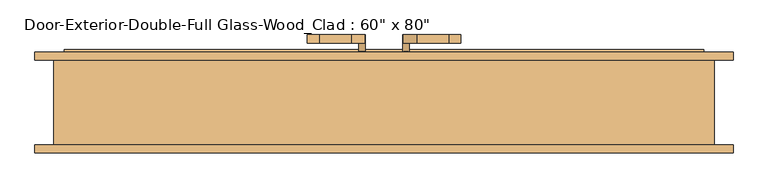
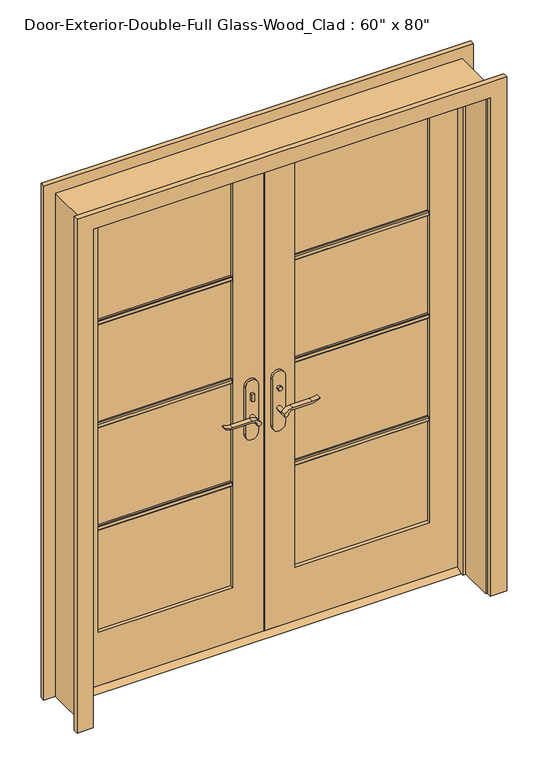
"""IFC4 building model written with IfcOpenShell, lengths in millimetres: door geometry."""

from ifc_helpers import new_model, si_unit, point, frame, frame_2d, origin, place, context, project, spatial, polyline, circle_curve, trimmed, segment, composite_curve, outline, extrude, faceted_brep, source, transform, mapped, element, save


def door_b03bd389(model_context):
    return source(origin(), model_context, "Body", "SolidModel", [
        extrude(outline(polyline([(63.5, 12.7), (98.425, 12.7), (123.825, 0.0), (38.1, 0.0), (63.5, 12.7)])), frame((-762.0, 0.0, 0.0), z_axis=(1.0, 0.0, 0.0), x_axis=(0.0, 1.0, 0.0)), (0.0, 0.0, 1.0), 1524.0),
        extrude(outline(polyline([(-47.4019111, 43.5), (-57.4019111, 43.5), (-57.4019111, 53.5), (-47.4019111, 53.5), (-47.4019111, 43.5)])), frame((0.0, 0.0, 981.9), z_axis=(0.0, 0.0, 1.0), x_axis=(1.0, 0.0, 0.0)), (0.0, 0.0, 1.0), 30.0),
        extrude(outline(composite_curve([segment(trimmed(circle_curve(frame_2d((996.9, -52.4019111)), 8.0), [point((996.9, -60.4019111))], [point((996.9, -44.4019111))], False, "CARTESIAN"), True, "CONTINUOUS"), segment(trimmed(circle_curve(frame_2d((996.9, -52.4019111)), 8.0), [point((996.9, -44.4019111))], [point((996.9, -60.4019111))], False, "CARTESIAN"), True, "CONTINUOUS")], self_intersect=False)), frame((0.0, 108.425, 0.0), z_axis=(0.0, 1.0, 0.0), x_axis=(0.0, 0.0, 1.0)), (0.0, 0.0, 1.0), 10.0),
        extrude(outline(composite_curve([segment(trimmed(circle_curve(frame_2d((897.1555521, -76.0694241)), 37.2832219), [point((919.0523287, -45.8937749))], [point((934.4, -77.7693445))], False, "CARTESIAN"), True, "CONTINUOUS"), segment(polyline([(934.4, -77.7693445), (934.4, -154.045502)]), True, "CONTINUOUS"), segment(trimmed(circle_curve(frame_2d((1017.6850638, -153.9791202)), 83.2850902), [point((934.4, -154.045502))], [point((939.4, -182.4019111))], True, "CARTESIAN"), True, "CONTINUOUS"), segment(polyline([(939.4, -182.4019111), (936.6135558, -182.4019111)]), True, "CONTINUOUS"), segment(trimmed(circle_curve(frame_2d((986.6709207, -150.4622499)), 59.3791355), [point((936.6135558, -182.4019111))], [point((927.4, -154.045502))], False, "CARTESIAN"), True, "CONTINUOUS"), segment(polyline([(927.4, -154.045502), (927.4, -77.7881013)]), True, "CONTINUOUS"), segment(trimmed(circle_curve(frame_2d((909.2738613, -77.7881013)), 18.1261387), [point((927.4, -77.7881013))], [point((914.4, -60.4019111))], True, "CARTESIAN"), True, "CONTINUOUS"), segment(trimmed(circle_curve(frame_2d((914.4, -52.4019111)), 8.0), [point((914.4, -60.4019111))], [point((919.0523287, -45.8937749))], False, "CARTESIAN"), True, "CONTINUOUS")], self_intersect=False)), frame((0.0, 3.5, 0.0), z_axis=(0.0, 1.0, 0.0), x_axis=(0.0, 0.0, 1.0)), (0.0, 0.0, 1.0), 20.0),
        extrude(outline(composite_curve([segment(trimmed(circle_curve(frame_2d((914.4, -52.4019111)), 8.0), [point((914.3999903, -60.4019111))], [point((919.0523287, -45.8937749))], False, "CARTESIAN"), True, "CONTINUOUS"), segment(trimmed(circle_curve(frame_2d((897.1555521, -76.0694241)), 37.2832219), [point((919.0523287, -45.8937749))], [point((934.4, -77.7693445))], False, "CARTESIAN"), True, "CONTINUOUS"), segment(polyline([(934.4, -77.7693445), (934.4, -154.045502)]), True, "CONTINUOUS"), segment(trimmed(circle_curve(frame_2d((1017.6850638, -153.9791202)), 83.2850902), [point((934.4, -154.045502))], [point((939.4, -182.4019111))], True, "CARTESIAN"), True, "CONTINUOUS"), segment(polyline([(939.4, -182.4019111), (936.6135558, -182.4019111)]), True, "CONTINUOUS"), segment(trimmed(circle_curve(frame_2d((986.6709207, -150.4622499)), 59.3791355), [point((936.6135558, -182.4019111))], [point((927.4, -154.045502))], False, "CARTESIAN"), True, "CONTINUOUS"), segment(polyline([(927.4, -154.045502), (927.4, -77.788099)]), True, "CONTINUOUS"), segment(trimmed(circle_curve(frame_2d((909.2738682, -77.788099)), 18.1261318), [point((927.4, -77.788099))], [point((914.3999903, -60.4019111))], True, "CARTESIAN"), True, "CONTINUOUS")], self_intersect=False)), frame((0.0, 138.425, 0.0), z_axis=(0.0, 1.0, 0.0), x_axis=(0.0, 0.0, 1.0)), (0.0, 0.0, 1.0), 20.0),
        extrude(outline(composite_curve([segment(trimmed(circle_curve(frame_2d((914.4, -52.4019111)), 8.0), [point((914.4, -60.4019111))], [point((914.4, -44.4019111))], False, "CARTESIAN"), True, "CONTINUOUS"), segment(trimmed(circle_curve(frame_2d((914.4, -52.4019111)), 8.0), [point((914.4, -44.4019111))], [point((914.4, -60.4019111))], False, "CARTESIAN"), True, "CONTINUOUS")], self_intersect=False)), frame((0.0, 23.5, 0.0), z_axis=(0.0, 1.0, 0.0), x_axis=(0.0, 0.0, 1.0)), (0.0, 0.0, 1.0), 30.0),
        extrude(outline(composite_curve([segment(trimmed(circle_curve(frame_2d((914.4, -52.4019111)), 8.0), [point((914.4, -60.4019111))], [point((914.4, -44.4019111))], False, "CARTESIAN"), True, "CONTINUOUS"), segment(trimmed(circle_curve(frame_2d((914.4, -52.4019111)), 8.0), [point((914.4, -44.4019111))], [point((914.4, -60.4019111))], False, "CARTESIAN"), True, "CONTINUOUS")], self_intersect=False)), frame((0.0, 108.425, 0.0), z_axis=(0.0, 1.0, 0.0), x_axis=(0.0, 0.0, 1.0)), (0.0, 0.0, 1.0), 30.0),
        extrude(outline(composite_curve([segment(polyline([(844.4, -27.4019111), (1039.4, -27.4019111)]), True, "CONTINUOUS"), segment(trimmed(circle_curve(frame_2d((1039.4, -52.4019111)), 25.0), [point((1039.4, -27.4019111))], [point((1039.4, -77.4019111))], False, "CARTESIAN"), True, "CONTINUOUS"), segment(polyline([(1039.4, -77.4019111), (844.4, -77.4019111)]), True, "CONTINUOUS"), segment(trimmed(circle_curve(frame_2d((844.4, -52.4019111)), 25.0), [point((844.4, -77.4019111))], [point((844.4, -27.4019111))], False, "CARTESIAN"), True, "CONTINUOUS")], self_intersect=False)), frame((0.0, 53.5, 0.0), z_axis=(0.0, 1.0, 0.0), x_axis=(0.0, 0.0, 1.0)), (0.0, 0.0, 1.0), 10.0),
        extrude(outline(composite_curve([segment(polyline([(844.4, -27.4019111), (1039.4, -27.4019111)]), True, "CONTINUOUS"), segment(trimmed(circle_curve(frame_2d((1039.4, -52.4019111)), 25.0), [point((1039.4, -27.4019111))], [point((1039.4, -77.4019111))], False, "CARTESIAN"), True, "CONTINUOUS"), segment(polyline([(1039.4, -77.4019111), (844.4, -77.4019111)]), True, "CONTINUOUS"), segment(trimmed(circle_curve(frame_2d((844.4, -52.4019111)), 25.0), [point((844.4, -77.4019111))], [point((844.4, -27.4019111))], False, "CARTESIAN"), True, "CONTINUOUS")], self_intersect=False)), frame((0.0, 98.425, 0.0), z_axis=(0.0, 1.0, 0.0), x_axis=(0.0, 0.0, 1.0)), (0.0, 0.0, 1.0), 10.0),
        extrude(outline(polyline([(47.3875, 118.425), (57.3875, 118.425), (57.3875, 108.425), (47.3875, 108.425), (47.3875, 118.425)])), frame((0.0, 0.0, 981.9), z_axis=(0.0, 0.0, 1.0), x_axis=(1.0, 0.0, 0.0)), (0.0, 0.0, 1.0), 30.0),
        extrude(outline(composite_curve([segment(trimmed(circle_curve(frame_2d((996.9, 52.3875)), 8.0), [point((996.9, 60.3875))], [point((996.9, 44.3875))], False, "CARTESIAN"), True, "CONTINUOUS"), segment(trimmed(circle_curve(frame_2d((996.9, 52.3875)), 8.0), [point((996.9, 44.3875))], [point((996.9, 60.3875))], False, "CARTESIAN"), True, "CONTINUOUS")], self_intersect=False)), frame((0.0, 43.5, 0.0), z_axis=(0.0, 1.0, 0.0), x_axis=(0.0, 0.0, 1.0)), (0.0, 0.0, 1.0), 10.0),
        extrude(outline(composite_curve([segment(trimmed(circle_curve(frame_2d((914.4, 52.3875)), 8.0), [point((919.0523287, 45.8793637))], [point((914.4, 60.3875))], False, "CARTESIAN"), True, "CONTINUOUS"), segment(trimmed(circle_curve(frame_2d((909.2738613, 77.7736901)), 18.1261387), [point((914.4, 60.3875))], [point((927.4, 77.7736901))], True, "CARTESIAN"), True, "CONTINUOUS"), segment(polyline([(927.4, 77.7736901), (927.4, 154.0310909)]), True, "CONTINUOUS"), segment(trimmed(circle_curve(frame_2d((986.6709207, 150.4478388)), 59.3791355), [point((927.4, 154.0310909))], [point((936.6135558, 182.3875))], False, "CARTESIAN"), True, "CONTINUOUS"), segment(polyline([(936.6135558, 182.3875), (939.4, 182.3875)]), True, "CONTINUOUS"), segment(trimmed(circle_curve(frame_2d((1017.6850638, 153.9647091)), 83.2850902), [point((939.4, 182.3875))], [point((934.4, 154.0310909))], True, "CARTESIAN"), True, "CONTINUOUS"), segment(polyline([(934.4, 154.0310909), (934.4, 77.7549333)]), True, "CONTINUOUS"), segment(trimmed(circle_curve(frame_2d((897.1555521, 76.0550129)), 37.2832219), [point((934.4, 77.7549333))], [point((919.0523287, 45.8793637))], False, "CARTESIAN"), True, "CONTINUOUS")], self_intersect=False)), frame((0.0, 138.425, 0.0), z_axis=(0.0, 1.0, 0.0), x_axis=(0.0, 0.0, 1.0)), (0.0, 0.0, 1.0), 20.0),
        extrude(outline(composite_curve([segment(trimmed(circle_curve(frame_2d((909.2738682, 77.7736878)), 18.1261318), [point((914.3999903, 60.3875))], [point((927.4, 77.7736878))], True, "CARTESIAN"), True, "CONTINUOUS"), segment(polyline([(927.4, 77.7736878), (927.4, 154.0310909)]), True, "CONTINUOUS"), segment(trimmed(circle_curve(frame_2d((986.6709207, 150.4478388)), 59.3791355), [point((927.4, 154.0310909))], [point((936.6135558, 182.3875))], False, "CARTESIAN"), True, "CONTINUOUS"), segment(polyline([(936.6135558, 182.3875), (939.4, 182.3875)]), True, "CONTINUOUS"), segment(trimmed(circle_curve(frame_2d((1017.6850638, 153.9647091)), 83.2850902), [point((939.4, 182.3875))], [point((934.4, 154.0310909))], True, "CARTESIAN"), True, "CONTINUOUS"), segment(polyline([(934.4, 154.0310909), (934.4, 77.7549333)]), True, "CONTINUOUS"), segment(trimmed(circle_curve(frame_2d((897.1555521, 76.0550129)), 37.2832219), [point((934.4, 77.7549333))], [point((919.0523287, 45.8793637))], False, "CARTESIAN"), True, "CONTINUOUS"), segment(trimmed(circle_curve(frame_2d((914.4, 52.3875)), 8.0), [point((919.0523287, 45.8793637))], [point((914.3999903, 60.3875))], False, "CARTESIAN"), True, "CONTINUOUS")], self_intersect=False)), frame((0.0, 3.5, 0.0), z_axis=(0.0, 1.0, 0.0), x_axis=(0.0, 0.0, 1.0)), (0.0, 0.0, 1.0), 20.0),
        extrude(outline(composite_curve([segment(trimmed(circle_curve(frame_2d((914.4, 52.3875)), 8.0), [point((914.4, 60.3875))], [point((914.4, 44.3875))], False, "CARTESIAN"), True, "CONTINUOUS"), segment(trimmed(circle_curve(frame_2d((914.4, 52.3875)), 8.0), [point((914.4, 44.3875))], [point((914.4, 60.3875))], False, "CARTESIAN"), True, "CONTINUOUS")], self_intersect=False)), frame((0.0, 108.425, 0.0), z_axis=(0.0, 1.0, 0.0), x_axis=(0.0, 0.0, 1.0)), (0.0, 0.0, 1.0), 30.0),
        extrude(outline(composite_curve([segment(trimmed(circle_curve(frame_2d((914.4, 52.3875)), 8.0), [point((914.4, 60.3875))], [point((914.4, 44.3875))], False, "CARTESIAN"), True, "CONTINUOUS"), segment(trimmed(circle_curve(frame_2d((914.4, 52.3875)), 8.0), [point((914.4, 44.3875))], [point((914.4, 60.3875))], False, "CARTESIAN"), True, "CONTINUOUS")], self_intersect=False)), frame((0.0, 23.5, 0.0), z_axis=(0.0, 1.0, 0.0), x_axis=(0.0, 0.0, 1.0)), (0.0, 0.0, 1.0), 30.0),
        extrude(outline(composite_curve([segment(trimmed(circle_curve(frame_2d((844.4, 52.3875)), 25.0), [point((844.4, 27.3875))], [point((844.4, 77.3875))], False, "CARTESIAN"), True, "CONTINUOUS"), segment(polyline([(844.4, 77.3875), (1039.4, 77.3875)]), True, "CONTINUOUS"), segment(trimmed(circle_curve(frame_2d((1039.4, 52.3875)), 25.0), [point((1039.4, 77.3875))], [point((1039.4, 27.3875))], False, "CARTESIAN"), True, "CONTINUOUS"), segment(polyline([(1039.4, 27.3875), (844.4, 27.3875)]), True, "CONTINUOUS")], self_intersect=False)), frame((0.0, 98.425, 0.0), z_axis=(0.0, 1.0, 0.0), x_axis=(0.0, 0.0, 1.0)), (0.0, 0.0, 1.0), 10.0),
        extrude(outline(composite_curve([segment(trimmed(circle_curve(frame_2d((844.4, 52.3875)), 25.0), [point((844.4, 27.3875))], [point((844.4, 77.3875))], False, "CARTESIAN"), True, "CONTINUOUS"), segment(polyline([(844.4, 77.3875), (1039.4, 77.3875)]), True, "CONTINUOUS"), segment(trimmed(circle_curve(frame_2d((1039.4, 52.3875)), 25.0), [point((1039.4, 77.3875))], [point((1039.4, 27.3875))], False, "CARTESIAN"), True, "CONTINUOUS"), segment(polyline([(1039.4, 27.3875), (844.4, 27.3875)]), True, "CONTINUOUS")], self_intersect=False)), frame((0.0, 53.5, 0.0), z_axis=(0.0, 1.0, 0.0), x_axis=(0.0, 0.0, 1.0)), (0.0, 0.0, 1.0), 10.0),
        extrude(outline(polyline([(77.47, 1502.171875), (77.47, 1483.121875), (71.12, 1483.121875), (67.945, 1486.296875), (67.945, 1498.996875), (71.12, 1502.171875), (77.47, 1502.171875)])), frame((120.65, 0.0, 0.0), z_axis=(1.0, 0.0, 0.0), x_axis=(0.0, 1.0, 0.0)), (0.0, 0.0, 1.0), 520.7),
        extrude(outline(polyline([(77.47, 1081.88125), (77.47, 1062.83125), (71.12, 1062.83125), (67.945, 1066.00625), (67.945, 1078.70625), (71.12, 1081.88125), (77.47, 1081.88125)])), frame((120.65, 0.0, 0.0), z_axis=(1.0, 0.0, 0.0), x_axis=(0.0, 1.0, 0.0)), (0.0, 0.0, 1.0), 520.7),
        extrude(outline(polyline([(77.47, 661.590625), (77.47, 642.540625), (71.12, 642.540625), (67.945, 645.715625), (67.945, 658.415625), (71.12, 661.590625), (77.47, 661.590625)])), frame((120.65, 0.0, 0.0), z_axis=(1.0, 0.0, 0.0), x_axis=(0.0, 1.0, 0.0)), (0.0, 0.0, 1.0), 520.7),
        extrude(outline(polyline([(84.455, 1502.171875), (90.805, 1502.171875), (93.98, 1498.996875), (93.98, 1486.296875), (90.805, 1483.121875), (84.455, 1483.121875), (84.455, 1502.171875)])), frame((-641.35, 0.0, 0.0), z_axis=(1.0, 0.0, 0.0), x_axis=(0.0, 1.0, 0.0)), (0.0, 0.0, 1.0), 520.7),
        extrude(outline(polyline([(84.455, 1081.88125), (90.805, 1081.88125), (93.98, 1078.70625), (93.98, 1066.00625), (90.805, 1062.83125), (84.455, 1062.83125), (84.455, 1081.88125)])), frame((-641.35, 0.0, 0.0), z_axis=(1.0, 0.0, 0.0), x_axis=(0.0, 1.0, 0.0)), (0.0, 0.0, 1.0), 520.7),
        extrude(outline(polyline([(84.455, 661.590625), (90.805, 661.590625), (93.98, 658.415625), (93.98, 645.715625), (90.805, 642.540625), (84.455, 642.540625), (84.455, 661.590625)])), frame((-641.35, 0.0, 0.0), z_axis=(1.0, 0.0, 0.0), x_axis=(0.0, 1.0, 0.0)), (0.0, 0.0, 1.0), 520.7),
        extrude(outline(polyline([(84.455, 1502.171875), (90.805, 1502.171875), (93.98, 1498.996875), (93.98, 1486.296875), (90.805, 1483.121875), (84.455, 1483.121875), (84.455, 1502.171875)])), frame((120.65, 0.0, 0.0), z_axis=(1.0, 0.0, 0.0), x_axis=(0.0, 1.0, 0.0)), (0.0, 0.0, 1.0), 520.7),
        extrude(outline(polyline([(84.455, 1081.88125), (90.805, 1081.88125), (93.98, 1078.70625), (93.98, 1066.00625), (90.805, 1062.83125), (84.455, 1062.83125), (84.455, 1081.88125)])), frame((120.65, 0.0, 0.0), z_axis=(1.0, 0.0, 0.0), x_axis=(0.0, 1.0, 0.0)), (0.0, 0.0, 1.0), 520.7),
        extrude(outline(polyline([(84.455, 661.590625), (90.805, 661.590625), (93.98, 658.415625), (93.98, 645.715625), (90.805, 642.540625), (84.455, 642.540625), (84.455, 661.590625)])), frame((120.65, 0.0, 0.0), z_axis=(1.0, 0.0, 0.0), x_axis=(0.0, 1.0, 0.0)), (0.0, 0.0, 1.0), 520.7),
        extrude(outline(polyline([(77.47, 1502.171875), (77.47, 1483.121875), (71.12, 1483.121875), (67.945, 1486.296875), (67.945, 1498.996875), (71.12, 1502.171875), (77.47, 1502.171875)])), frame((-641.35, 0.0, 0.0), z_axis=(1.0, 0.0, 0.0), x_axis=(0.0, 1.0, 0.0)), (0.0, 0.0, 1.0), 520.7),
        extrude(outline(polyline([(77.47, 1081.88125), (77.47, 1062.83125), (71.12, 1062.83125), (67.945, 1066.00625), (67.945, 1078.70625), (71.12, 1081.88125), (77.47, 1081.88125)])), frame((-641.35, 0.0, 0.0), z_axis=(1.0, 0.0, 0.0), x_axis=(0.0, 1.0, 0.0)), (0.0, 0.0, 1.0), 520.7),
        extrude(outline(polyline([(77.47, 661.590625), (77.47, 642.540625), (71.12, 642.540625), (67.945, 645.715625), (67.945, 658.415625), (71.12, 661.590625), (77.47, 661.590625)])), frame((-641.35, 0.0, 0.0), z_axis=(1.0, 0.0, 0.0), x_axis=(0.0, 1.0, 0.0)), (0.0, 0.0, 1.0), 520.7),
        extrude(outline(polyline([(0.0, 768.35), (0.0, 831.85), (2101.85, 831.85), (2101.85, -831.85), (0.0, -831.85), (0.0, -768.35), (2038.35, -768.35), (2038.35, 768.35), (0.0, 768.35)])), frame((0.0, 98.425, 0.0), z_axis=(0.0, 1.0, 0.0), x_axis=(0.0, 0.0, 1.0)), (0.0, 0.0, 1.0), 19.05),
        extrude(outline(polyline([(0.0, 768.35), (0.0, 831.85), (2101.85, 831.85), (2101.85, -831.85), (0.0, -831.85), (0.0, -768.35), (2038.35, -768.35), (2038.35, 768.35), (0.0, 768.35)])), frame((0.0, -123.825, 0.0), z_axis=(0.0, 1.0, 0.0), x_axis=(0.0, 0.0, 1.0)), (0.0, 0.0, 1.0), 19.05),
        extrude(outline(polyline([(12.7, 762.0), (2032.0, 762.0), (2032.0, 1.5875), (12.7, 1.5875), (12.7, 762.0)]), holes=[polyline([(1912.9375, 120.65), (1912.9375, 641.35), (231.775, 641.35), (231.775, 120.65), (1912.9375, 120.65)])]), frame((0.0, 63.5, 0.0), z_axis=(0.0, 1.0, 0.0), x_axis=(0.0, 0.0, 1.0)), (0.0, 0.0, 1.0), 34.925),
        extrude(outline(polyline([(2032.0, -762.0), (12.7, -762.0), (12.7, -1.6019111), (2032.0, -1.6019111), (2032.0, -762.0)]), holes=[polyline([(231.775, -641.35), (1912.9375, -641.35), (1912.9375, -120.65), (231.775, -120.65), (231.775, -641.35)])]), frame((0.0, 63.5, 0.0), z_axis=(0.0, 1.0, 0.0), x_axis=(0.0, 0.0, 1.0)), (0.0, 0.0, 1.0), 34.925),
        faceted_brep([(787.4, 98.425, 0.0), (787.4, -104.775, 0.0), (762.0, -104.775, 0.0), (762.0, 28.575, 0.0), (749.3, 28.575, 0.0), (749.3, 63.5, 0.0), (762.0, 63.5, 0.0), (762.0, 98.425, 0.0), (787.4, 98.425, 2057.4), (787.4, -104.775, 2057.4), (-787.4, -104.775, 2057.4), (-787.4, -104.775, 0.0), (-762.0, -104.775, 0.0), (-762.0, -104.775, 2032.0), (762.0, -104.775, 2032.0), (762.0, 28.575, 2032.0), (-762.0, 28.575, 2032.0), (-762.0, 28.575, 0.0), (-749.3, 28.575, 0.0), (-749.3, 28.575, 2019.3), (749.3, 28.575, 2019.3), (749.3, 63.5, 2019.3), (1.5875, 63.5, 2019.3), (-1.6019111, 63.5, 2019.3), (-749.3, 63.5, 2019.3), (-749.3, 63.5, 0.0), (-762.0, 63.5, 0.0), (-762.0, 63.5, 2032.0), (-1.6019111, 63.5, 2032.0), (1.5875, 63.5, 2032.0), (762.0, 63.5, 2032.0), (762.0, 98.425, 2032.0), (1.5875, 98.425, 2032.0), (-1.6019111, 98.425, 2032.0), (-762.0, 98.425, 2032.0), (-762.0, 98.425, 0.0), (-787.4, 98.425, 0.0), (-787.4, 98.425, 2057.4)], [[[0, 1, 2, 3, 4, 5, 6, 7]], [[1, 0, 8, 9]], [[2, 1, 9, 10, 11, 12, 13, 14]], [[3, 2, 14, 15]], [[4, 3, 15, 16, 17, 18, 19, 20]], [[5, 4, 20, 21]], [[6, 5, 21, 22, 23, 24, 25, 26, 27, 28, 29, 30]], [[7, 6, 30, 31]], [[0, 7, 31, 32, 33, 34, 35, 36, 37, 8]], [[9, 8, 37, 10]], [[14, 13, 16, 15]], [[20, 19, 24, 23, 22, 21]], [[31, 30, 29, 28, 27, 34, 33, 32]], [[12, 11, 36, 35, 26, 25, 18, 17]], [[11, 10, 37, 36]], [[13, 12, 17, 16]], [[19, 18, 25, 24]], [[27, 26, 35, 34]]]),
        extrude(outline(polyline([(641.35, 77.47), (120.65, 77.47), (120.65, 84.455), (641.35, 84.455), (641.35, 77.47)])), frame((0.0, 0.0, 231.775), z_axis=(0.0, 0.0, 1.0), x_axis=(1.0, 0.0, 0.0)), (0.0, 0.0, 1.0), 1681.1625),
        extrude(outline(polyline([(-120.65, 77.47), (-641.35, 77.47), (-641.35, 84.455), (-120.65, 84.455), (-120.65, 77.47)])), frame((0.0, 0.0, 231.775), z_axis=(0.0, 0.0, 1.0), x_axis=(1.0, 0.0, 0.0)), (0.0, 0.0, 1.0), 1681.1625),
    ])


if __name__ == "__main__":
    model = new_model("IFC4")
    model_context = context("Model", 3, world=origin())
    ifc_project = project(units=[si_unit("LENGTHUNIT", "METRE", prefix="MILLI")], contexts=[model_context])
    site = spatial("IfcSite", under=ifc_project)
    building = spatial("IfcBuilding", under=site)
    placement = place(None, origin())
    door_shape = door_b03bd389(model_context)
    element("IfcDoor", 1, ObjectType="Door-Exterior-Double-Full Glass-Wood_Clad : 60\" x 80\"", at=placement, inside=building, context=model_context, shape_type="MappedRepresentation", body=[
        mapped(door_shape, transform((0.0, 0.0, 0.0), x_axis=(1.0, 0.0, 0.0), y_axis=(0.0, 1.0, 0.0), z_axis=(0.0, 0.0, 1.0))),
    ])
    save(model, "model.ifc")

# Revit data of these elements
# Type "Door-Exterior-Double-Full Glass-Wood_Clad : 60\" x 80\""
#   Type Mark = "18"
#   Assembly Code = "B2030100"
#   Analytic Construction = "French door, wood frame with double glass"
#   Top Rail = 0' - 4 11/16"
#   Threshold Offset [instance default] = 0' - 0 1/2"
#   Thickness = 0' - 1 3/8"
#   Thermal Resistance (R) = 1.9158 (h·ft²·°F)/BTU
#   Swing Angle [instance default] = 90.00°
#   Stiles = 0' - 4 3/4"
#   Rough Width = 5' - 2"
#   Rough Height = 6' - 9"
#   Panel Width = 2' - 6"
#   Door Offset [instance default] = 0' - 0"
#   Height = 6' - 8"
#   Width = 5' - 0"
#   Heat Transfer Coefficient (U) = 0.5220 BTU/(h·ft²·°F)
#   Bottom Rail = 0' - 9 1/8"
#   Exterior Trim [instance default] = yes
#   Threshold [instance default] = yes
#   Show Grill [instance default] = yes
#   Function = 1
#   Trim Material = Cherry
#   Threshold Material = Cherry
#   Panel Material = Cherry
#   Glazing = Glass
#   Frame Material = Cherry
#   Door Handle Material = Aluminum
#   Visual Light Transmittance = 0
#   Solar Heat Gain Coefficient = 0
#   Wall Closure = (empty or 0)
#   Construction Type = (empty or 0)
# Element 1 (IfcDoor, "Door-Exterior-Double-Full Glass-Wood_Clad : 60\" x 80\"")
#   Materials on its faces: "Cherry", "Aluminum", "Glass"
# Materials
#   "Cherry": class "Wood", colour RGB 226 177 128, transparency 0, Description = "Prunus Serotina", Cost = 0
#   "Glass": class "Glass", colour RGB 0 128 192, transparency 0.75, Description = "Soda Lime Glass", Cost = 0
#   "Aluminum": class "Metal", colour RGB 247 247 247, transparency 0, Description = "Aluminum 6061", Cost = 0
